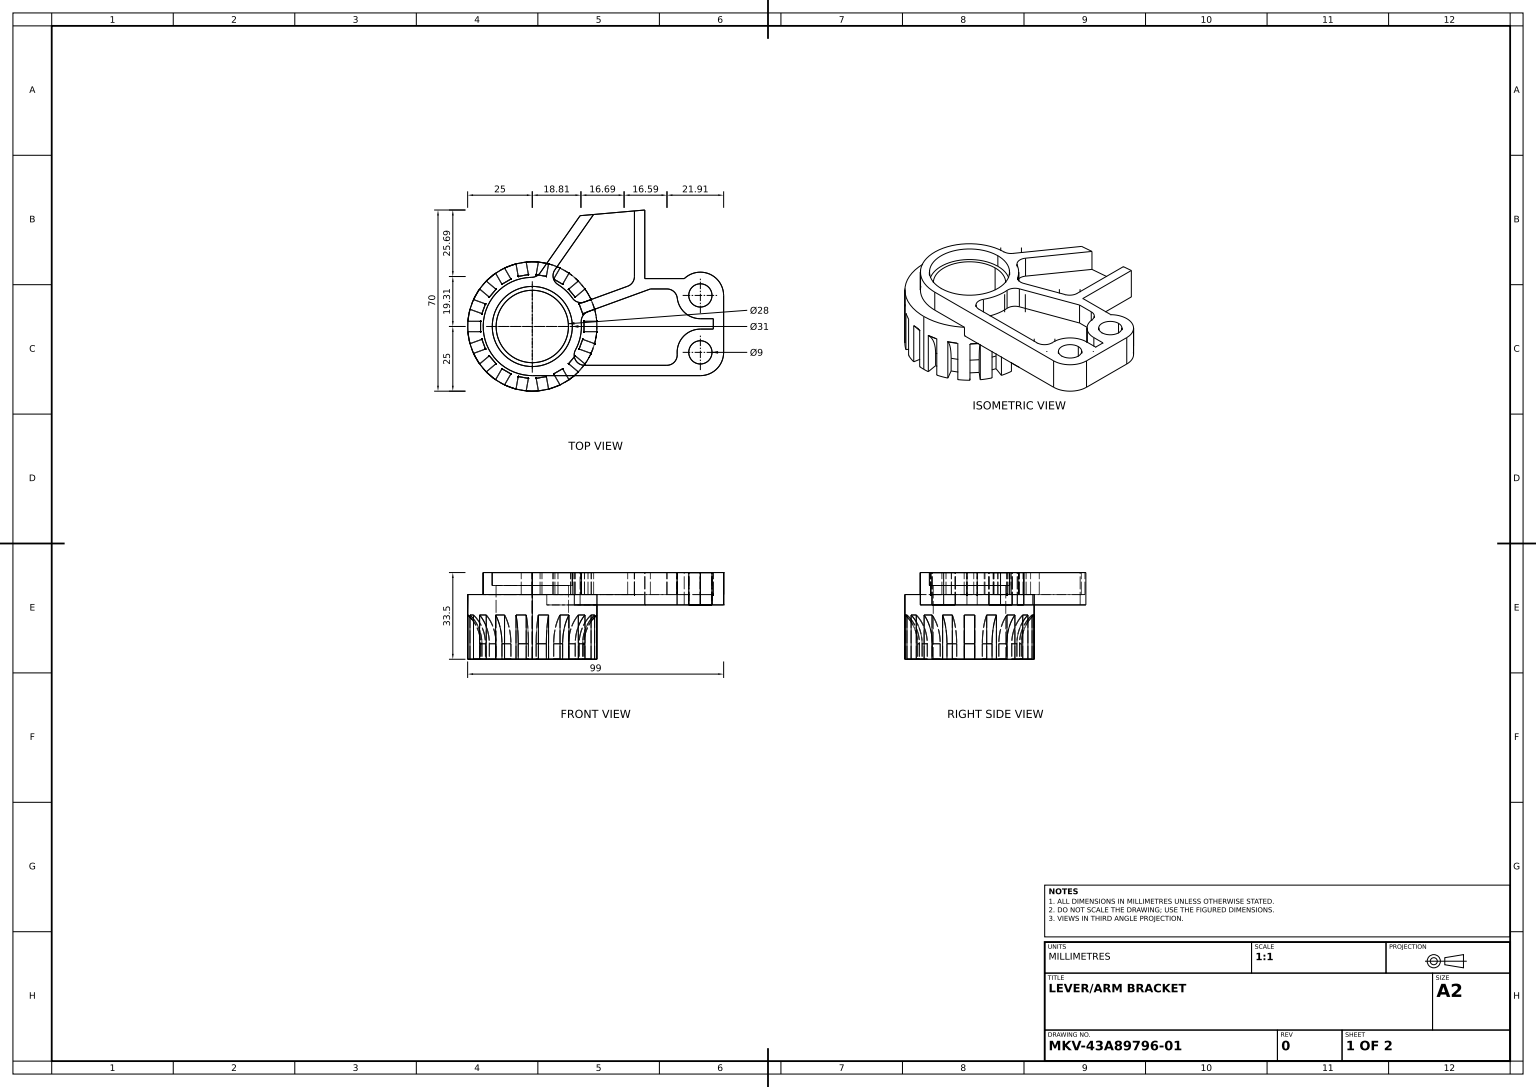
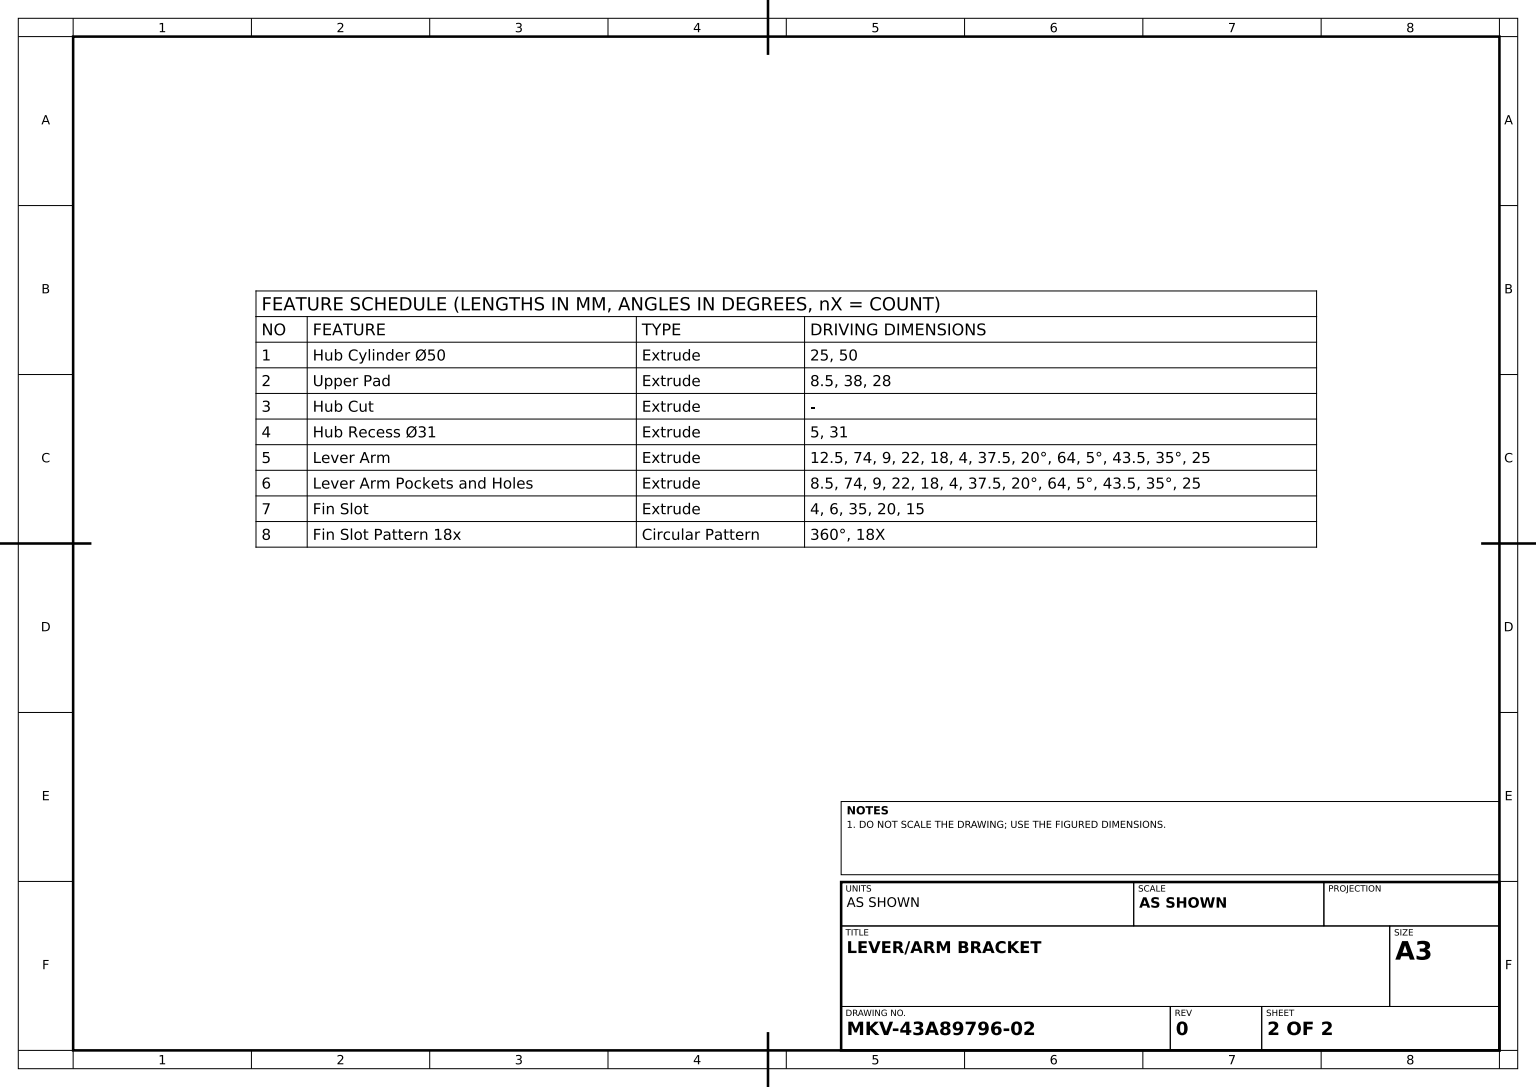
from build123d import *

# Parameters (mm, degrees)
HUB_SKETCH_50_R                   = 25
HUB_CYLINDER_50_DEPTH             = 25
UPPER_PAD_SKETCH_R                = 19
UPPER_PAD_SKETCH_R_2              = 14
UPPER_PAD_DEPTH                   = 8.5
HUB_CUT_REACH                     = 45.301
HUB_CUT_SKETCH_R                  = 14
HUB_RECESS_SKETCH_31_R            = 15.5
HUB_RECESS_31_DEPTH               = 5
LEVER_START                       = -12.5
LEVER_ARM_PROFILE_SKETCH_R        = 4.5
LEVER_ARM_DEPTH                   = 12.5
LEVER_START_2                     = -8.5
LEVER_ARM_POCKETS_AND_HOLES_DEPTH = 8.5
FIN_SLOT_DEPTH                    = 2
FIN_SLOT_PATTERN_18X_COUNT        = 18


with BuildPart() as part:
    # Hub Sketch _50 → Hub Cylinder _50 (new body)
    with BuildSketch(Plane(origin=(0, 0, 0), x_dir=(1, 0, 0), z_dir=(0, 1, 0))):
        with Locations(Location((0, 0, 0), (0, 0, 270))):
            Circle(HUB_SKETCH_50_R)
    extrude(amount=-HUB_CYLINDER_50_DEPTH)

    # Upper Pad Sketch → Upper Pad (add)
    with BuildSketch(Plane(origin=(0, 0, 0), x_dir=(1, 0, 0), z_dir=(0, 1, 0))):
        with Locations(Location((0, 0, 0), (0, 0, 270))):
            Circle(UPPER_PAD_SKETCH_R)
        with Locations(Location((0, 0, 0), (0, 0, 270))):
            Circle(UPPER_PAD_SKETCH_R_2, mode=Mode.SUBTRACT)
    extrude(amount=UPPER_PAD_DEPTH)

    # Hub Cut Sketch → Hub Cut (cut, up to next)
    with BuildSketch(Plane(origin=(0, 0, 0), x_dir=(1, 0, 0), z_dir=(0, 1, 0)), mode=Mode.PRIVATE) as hub_cut_sk1:
        with Locations(Location((0, 0, 0), (0, 0, 270))):
            Circle(HUB_CUT_SKETCH_R)
    hub_cut_tool1 = extrude(hub_cut_sk1.sketch, amount=-HUB_CUT_REACH, mode=Mode.PRIVATE) & part.part
    add(hub_cut_tool1.solids().sort_by_distance((0, 0, 0))[0], mode=Mode.SUBTRACT)

    # Hub Recess Sketch _31 → Hub Recess _31 (cut)
    with BuildSketch(Plane(origin=(0, 8.5, 0), x_dir=(1, 0, 0), z_dir=(0, 1, 0))):
        with Locations(Location((0, 0, 0), (0, 0, 270))):
            Circle(HUB_RECESS_SKETCH_31_R)
    extrude(amount=-HUB_RECESS_31_DEPTH, mode=Mode.SUBTRACT)

    # Lever Arm Profile Sketch → Lever Arm (add)
    with BuildSketch(Plane(origin=(0, 8.5, 0), x_dir=(1, 0, 0), z_dir=(0, 1, 0)).offset(LEVER_START)):
        with BuildLine():
            Line((0, -19), (65, -19))
            ThreePointArc((65, -19), (71.363961031, -16.363961031), (74, -10))
            Line((74, -10), (74, 12))
            ThreePointArc((74, 12), (68.53379766, 20.277214151), (58.775050201, 18.5))
            Line((58.775050201, 18.5), (43.5, 18.5))
            Line((43.5, 18.5), (43.5, 45))
            Line((43.5, 45), (18.5, 42.812783412))
            Line((18.5, 42.812783412), (3.019442807, 20.704256513))
            ThreePointArc((3.019442807, 20.704256513), (1.609636047, 19.460900253), (-0.212440958, 18.998812301))
            ThreePointArc((-0.212440958, 18.998812301), (18.999703073, 0.106222139), (0, -19))
        make_face()
        with Locations(Location((65, -10, 0), (0, 0, 270))):
            Circle(LEVER_ARM_PROFILE_SKETCH_R, mode=Mode.SUBTRACT)
        with Locations(Location((65, 12, 0), (0, 0, 270))):
            Circle(LEVER_ARM_PROFILE_SKETCH_R, mode=Mode.SUBTRACT)
    extrude(amount=LEVER_ARM_DEPTH)

    # Sketch5_3 → Lever Arm Pockets and Holes (cut)
    with BuildSketch(Plane(origin=(0, 8.5, 0), x_dir=(1, 0, 0), z_dir=(0, 1, 0)).offset(LEVER_START_2)):
        with BuildLine():
            ThreePointArc((19, 0), (18.412450045, -4.688462793), (16.686138594, -9.086956522))
            ThreePointArc((16.686138594, -9.086956522), (16.760102062, -13.043015674), (20.199009877, -15))
            Line((20.199009877, -15), (52.038518603, -15))
            ThreePointArc((52.038518603, -15), (54.973716146, -13.717464882), (56.026666725, -10.692307692))
            ThreePointArc((56.026666725, -10.692307692), (58.395805529, -3.885704016), (65, -1))
            Line((65, -1), (70, -1))
            Line((70, -1), (70, 3))
            Line((70, 3), (65, 3))
            ThreePointArc((65, 3), (59.014440454, 5.278908056), (56.06011199, 10.961538462))
            ThreePointArc((56.06011199, 10.961538462), (54.747077117, 13.487151975), (52.08682843, 14.5))
            Line((52.08682843, 14.5), (45.686031382, 14.5))
            Line((45.686031382, 14.5), (21.548602473, 5.714694345))
            ThreePointArc((21.548602473, 5.714694345), (19.545401033, 4.1087029), (18.931172951, 1.61576319))
            ThreePointArc((18.931172951, 1.61576319), (18.982785439, 0.808614224), (19, 0))
        make_face()
        with BuildLine():
            ThreePointArc((8.742589, 21.903969159), (8.102979357, 18.795269171), (9.928902016, 16.199287168))
            ThreePointArc((9.928902016, 16.199287168), (13.004387246, 13.852289066), (15.5407124, 10.930976996))
            ThreePointArc((15.5407124, 10.930976996), (17.613669166, 9.416092585), (20.1805219, 9.473464828))
            Line((20.1805219, 9.473464828), (36.868080573, 15.547239468))
            ThreePointArc((36.868080573, 15.547239468), (38.776608177, 17.011704206), (39.5, 19.306009951))
            Line((39.5, 19.306009951), (39.5, 44.650045346))
            Line((39.5, 44.650045346), (23.701759282, 43.267878379))
            Line((23.701759282, 43.267878379), (8.742589, 21.903969159))
        make_face()
    extrude(amount=LEVER_ARM_POCKETS_AND_HOLES_DEPTH, mode=Mode.SUBTRACT)

    # Fin Slot Sketch → Fin Slot (cut, symmetric)
    with BuildSketch(Plane.XY):
        with BuildLine():
            Line((20, -25), (20, -19))
            ThreePointArc((20, -19), (21.306936062, -12.876275643), (25, -7.819660113))
            Line((25, -7.819660113), (25, -25))
            Line((25, -25), (20, -25))
        make_face()
    fin_slot = extrude(amount=FIN_SLOT_DEPTH, both=True, mode=Mode.SUBTRACT)

    # Fin Slot Pattern 18x: Fin Slot ×18 about axis
    fin_slot_pattern_18x_axis = Axis((0, 0, 0), (0, 1, 0))
    for i in range(1, FIN_SLOT_PATTERN_18X_COUNT):
        add(fin_slot.rotate(fin_slot_pattern_18x_axis, i * 360 / FIN_SLOT_PATTERN_18X_COUNT), mode=Mode.SUBTRACT)


solid = part.part
